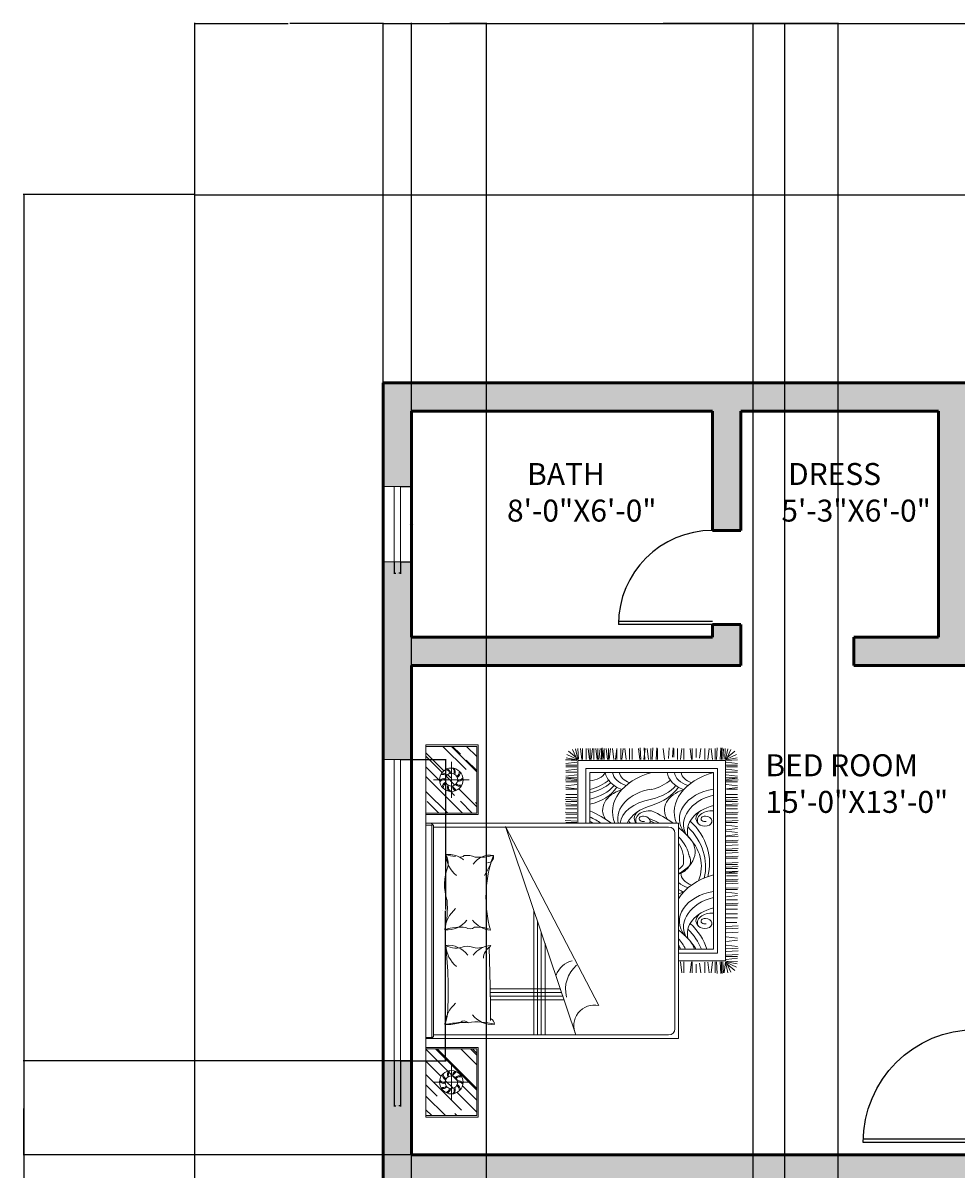
# Model space of a CAD drawing. Units: inches. Extents: x 134045 to 134755, y 144691 to 145880.
# Tile 4 of 6: x 134045 to 134343, y 145515 to 145880. Entities that reach past the tile are written whole.
import ezdxf

# ---------------------------------------------------------------- set-up
doc = ezdxf.new("R2010")
doc.units = ezdxf.units.IN
for name, color, linetype, lineweight in [('A-ANNO-DIMS', 2, 'Continuous', 18), ('A-AREA-IDEN', 7, 'Continuous', 18), ('A-DOOR', 4, 'Continuous', 25), ('A-FURN', 8, 'Continuous', 18), ('A-GLAZ', 4, 'Continuous', 18), ('A-WALL', 7, 'Continuous', 50), ('A-WALL-PATT', 252, 'Continuous', 13), ('C-PROP', 7, 'Continuous', 25)]:
    doc.layers.add(name, color=color, linetype=linetype, lineweight=lineweight)
doc.styles.get("Standard").update_dxf_attribs({"font": 'arial.ttf'})
doc.dimstyles.get("Standard").update_dxf_attribs({"dimtxt": 0.18, "dimasz": 0.18, "dimexe": 0.18, "dimexo": 0.0625, "dimgap": 0.09, "dimtad": 0, "dimtih": 1, "dimtoh": 1, "dimdec": 4, "dimzin": 0, "dimdsep": 46, "dimtxsty": 'Standard', "dimcen": 0.09, "dimadec": 0, "dimazin": 0, "dimtfac": 1, "dimtdec": 4, "dimtofl": 0, "dimtmove": 0, "dimatfit": 3, "dimfxl": 1, "dimtolj": 1, "dimtzin": 0, "dimarcsym": 0})

# ---------------------------------------------------------------- blocks, each defined once
blk = doc.blocks.new('A$C64B41DC1')
for p, q in [((0, 2.5079), (2.9903, 2.5079)), ((0, 2.0879), (0, 2.5079)), ((0.012, 2.4618), (0.0581, 2.5079)), ((0.012, 2.3515), (0.1684, 2.5079)), ((0.012, 2.0999), (0.012, 2.5079)), ((0.0543, 2.2213), (0.3409, 2.5079)), ((0.1689, 2.4179), (0.2589, 2.5079)), ((0.3265, 2.386), (0.4484, 2.5079)), ((0.3699, 2.3332), (0.5445, 2.5079)), ((0.548, 2.5079), (0.548, 2.0999)), ((0.56, 2.5079), (0.56, 2.0879)), ((0.6301, 2.5079), (0.6301, 0.4779)), ((0.6401, 2.461), (0.6401, 2.5079)), ((0.6401, 2.5079), (2.344, 2.5079)), ((2.344, 2.5079), (2.3601, 2.5079)), ((2.344, 2.5079), (2.344, 2.461)), ((2.3601, 2.5079), (2.3601, 2.4761)), ((2.3601, 0.4779), (2.3601, 2.5079)), ((2.4303, 2.5079), (2.4303, 2.0879)), ((2.4423, 2.5079), (2.4423, 2.0999)), ((2.4423, 2.3333), (2.6169, 2.5079)), ((2.4423, 2.2145), (2.7357, 2.5079)), ((2.4423, 2.404), (2.5354, 2.4971)), ((2.705, 2.398), (2.8149, 2.5079)), ((2.7691, 2.3772), (2.8998, 2.5079)), ((2.7819, 2.3646), (2.9252, 2.5079)), ((2.9783, 2.0999), (2.9783, 2.5079)), ((2.9903, 2.0879), (2.9903, 2.5079)), ((0.2157, 2.0999), (0.548, 2.4322)), ((0.2299, 2.0999), (0.548, 2.418)), ((0.2804, 2.1597), (0.2804, 2.4481)), ((2.344, 2.461), (0.6401, 2.461)), ((0.6601, 2.4461), (1.4951, 2.4461)), ((0.6601, 2.4461), (0.6601, 0.5579)), ((1.4951, 2.4461), (0.6697, 2.4461)), ((2.3301, 2.4461), (1.4951, 2.4461)), ((2.3301, 0.5579), (2.3301, 2.4461)), ((2.7099, 2.1597), (2.7099, 2.4481)), ((0.1362, 2.3039), (0.4246, 2.3039)), ((0.2311, 2.2906), (0.2937, 2.3532)), ((0.3405, 2.3039), (0.3605, 2.3238)), ((2.8541, 2.3039), (2.5657, 2.3039)), ((2.5849, 2.2779), (2.6158, 2.3088)), ((2.6158, 2.3088), (2.6313, 2.3243)), ((2.6674, 2.2756), (2.7382, 2.3464)), ((2.7249, 2.3076), (2.7512, 2.3339)), ((2.7746, 2.0999), (2.9783, 2.3036)), ((2.7914, 2.1846), (2.9783, 2.3715)), ((0.012, 2.261), (0.0275, 2.2765)), ((0.0404, 2.0999), (0.1982, 2.2578)), ((0.1365, 2.0999), (0.251, 2.2144)), ((0.2905, 2.2539), (0.3304, 2.2938)), ((0.4194, 2.0999), (0.548, 2.2285)), ((2.4423, 2.1353), (2.5382, 2.2312)), ((2.4918, 2.0999), (2.6366, 2.2447)), ((2.9144, 2.2312), (2.9783, 2.2951)), ((0.4986, 2.0999), (0.548, 2.1493)), ((0.5127, 2.0999), (0.548, 2.1352)), ((2.7831, 2.0999), (2.8678, 2.1846)), ((2.8962, 2.0999), (2.9783, 2.182)), ((0.56, 2.0879), (0, 2.0879)), ((0.548, 2.0999), (0.012, 2.0999)), ((2.4303, 2.0879), (2.9903, 2.0879)), ((2.4423, 2.0999), (2.9783, 2.0999)), ((2.5172, 2.0999), (2.5269, 2.1096)), ((0.9415, 1.9902), (0.9415, 1.3975)), ((0.9715, 1.9906), (0.9715, 1.4076)), ((1.0015, 1.991), (1.0015, 1.4177)), ((1.0315, 1.9916), (1.0315, 1.4279)), ((2.3349, 1.8678), (0.6613, 1.3029)), ((0.8956, 1.1191), (2.3349, 1.8678)), ((1.6636, 1.6412), (0.6601, 1.6412)), ((1.5748, 1.6112), (0.6601, 1.6112)), ((2.3665, 1.295), (2.3665, 1.3839)), ((2.377, 1.295), (2.3822, 1.3891)), ((2.4032, 1.295), (2.4032, 1.3839)), ((2.4346, 1.295), (2.4346, 1.3839)), ((2.4451, 1.295), (2.4503, 1.3891)), ((2.4774, 1.2957), (2.4774, 1.3837)), ((2.5, 1.295), (2.5, 1.3839)), ((2.5105, 1.295), (2.5157, 1.3891)), ((2.5367, 1.295), (2.5367, 1.3839)), ((2.5471, 1.295), (2.5524, 1.3891)), ((2.5681, 1.295), (2.5681, 1.3839)), ((2.5918, 1.295), (2.5918, 1.3839)), ((2.6346, 1.2957), (2.6346, 1.3837)), ((2.6362, 1.2957), (2.6467, 1.3839)), ((2.6729, 1.295), (2.6624, 1.3839)), ((2.6938, 1.295), (2.6938, 1.3839)), ((2.7043, 1.295), (2.7095, 1.3891)), ((2.7127, 1.2957), (2.7232, 1.3839)), ((2.7253, 1.295), (2.7253, 1.3839)), ((2.7494, 1.295), (2.7389, 1.3839)), ((2.7718, 1.295), (2.7718, 1.3839)), ((2.7959, 1.295), (2.7854, 1.3839)), ((2.8146, 1.2957), (2.8146, 1.3837)), ((2.8146, 1.2957), (2.8146, 1.3837)), ((2.8282, 1.295), (2.8282, 1.3839)), ((2.8282, 1.295), (2.8282, 1.3839)), ((2.8523, 1.295), (2.8418, 1.3839)), ((2.8523, 1.295), (2.8418, 1.3839)), ((2.8653, 1.2966), (2.8688, 1.3861)), ((2.8711, 1.2957), (2.8711, 1.3837)), ((2.8711, 1.2957), (2.8875, 1.3822)), ((2.8713, 1.2927), (2.954, 1.3315)), ((2.8717, 1.2884), (2.9588, 1.3058)), ((2.8765, 1.2958), (2.9132, 1.3758)), ((2.8893, 1.3011), (2.9394, 1.3636)), ((2.3601, 1.2873), (2.8639, 1.2873)), ((2.3601, 1.2233), (2.7999, 1.2233)), ((2.7999, 1.2233), (2.7999, 0.1658)), ((2.8639, 1.2873), (2.8639, 0.1018)), ((2.8716, 1.2565), (2.9605, 1.2669)), ((2.8716, 1.2212), (2.9605, 1.2212)), ((2.8716, 1.1947), (2.9605, 1.2052)), ((2.8723, 1.2489), (2.9603, 1.2489)), ((2.8744, 1.2817), (2.9603, 1.2869)), ((2.3601, 1.1913), (2.7679, 1.1912)), ((2.7679, 1.1912), (2.7679, 0.1978)), ((2.8716, 1.181), (2.9605, 1.1705)), ((2.8716, 1.1595), (2.9605, 1.1595)), ((2.8716, 1.133), (2.9605, 1.1435)), ((2.8716, 1.1193), (2.9605, 1.1088)), ((2.8723, 1.1872), (2.9603, 1.1872)), ((2.8723, 1.1255), (2.9603, 1.1255)), ((2.8716, 1.1035), (2.9605, 1.093)), ((2.8716, 1.0965), (2.9605, 1.0965)), ((2.8716, 1.086), (2.9657, 1.0913)), ((2.8716, 1.0756), (2.9605, 1.0756)), ((2.8716, 1.0491), (2.9605, 1.0596)), ((2.8716, 1.0354), (2.9605, 1.0249)), ((2.8723, 1.0858), (2.9605, 1.0753)), ((2.8723, 1.0416), (2.9603, 1.0416)), ((2.8716, 0.9346), (2.9605, 0.9241)), ((2.8723, 0.9987), (2.9605, 1.0092)), ((2.8723, 0.985), (2.9605, 0.9745)), ((2.8723, 0.9735), (2.9603, 0.9735)), ((2.8723, 0.9408), (2.9603, 0.9408)), ((2.8723, 0.8979), (2.9605, 0.9084)), ((2.8723, 0.8726), (2.9603, 0.8726)), ((2.8723, 0.8505), (2.9603, 0.8505)), ((2.8716, 0.7885), (2.9605, 0.799)), ((2.8716, 0.7818), (2.9657, 0.787)), ((2.8716, 0.7503), (2.9657, 0.7556)), ((2.8723, 0.7571), (2.9605, 0.7466)), ((2.8716, 0.7204), (2.9605, 0.7309)), ((2.8716, 0.6995), (2.9605, 0.6995)), ((2.8716, 0.689), (2.9657, 0.6838)), ((2.8716, 0.6576), (2.9657, 0.6523)), ((2.8716, 0.6471), (2.9605, 0.6471)), ((2.8716, 0.5903), (2.9605, 0.6007)), ((2.882, 0.5582), (2.9657, 0.5536)), ((0.6301, 0.4779), (2.3601, 0.4779)), ((0.7101, 0.5079), (2.2801, 0.5079)), ((1.2465, 0.4625), (1.1576, 0.452)), ((1.2542, 0.1018), (1.2542, 0.4779)), ((1.3182, 0.1658), (1.3182, 0.4779)), ((1.3502, 0.1978), (1.3502, 0.4779)), ((2.8716, 0.4877), (2.9603, 0.4877)), ((2.8716, 0.4625), (2.9605, 0.452)), ((2.8909, 0.5263), (2.9657, 0.5222)), ((2.8928, 0.5169), (2.9605, 0.5169)), ((1.2465, 0.3746), (1.1576, 0.3851)), ((1.2465, 0.4365), (1.1577, 0.4365)), ((1.2465, 0.3684), (1.1577, 0.3684)), ((2.8716, 0.4365), (2.9603, 0.4365)), ((2.8716, 0.3746), (2.9605, 0.3851)), ((2.8716, 0.3684), (2.9603, 0.3684)), ((1.2355, 0.3092), (1.1576, 0.3)), ((1.2285, 0.3357), (1.1577, 0.3357)), ((2.8826, 0.3092), (2.9605, 0.3)), ((2.8896, 0.3357), (2.9603, 0.3357)), ((1.2457, 0.2423), (1.1576, 0.2319)), ((1.2465, 0.2057), (1.1576, 0.2161)), ((1.2465, 0.1847), (1.1576, 0.1847)), ((1.2457, 0.2676), (1.1577, 0.2676)), ((2.7679, 0.1978), (1.3502, 0.1978)), ((2.8716, 0.2057), (2.9605, 0.2161)), ((2.8716, 0.1847), (2.9605, 0.1847)), ((2.8723, 0.2676), (2.9603, 0.2676)), ((2.8723, 0.2423), (2.9605, 0.2319)), ((1.2465, 0.1742), (1.1524, 0.169)), ((1.2465, 0.1428), (1.1524, 0.1376)), ((1.2465, 0.1334), (1.1524, 0.1281)), ((1.2465, 0.1323), (1.1576, 0.1323)), ((1.2465, 0.1323), (1.1576, 0.1323)), ((1.2465, 0.1), (1.1576, 0.1105)), ((1.2465, 0.1229), (1.1588, 0.1168)), ((1.2464, 0.1007), (1.1592, 0.0833)), ((1.2468, 0.0964), (1.1641, 0.0576)), ((1.2415, 0.0933), (1.2049, 0.0133)), ((1.247, 0.0934), (1.2306, 0.0069)), ((1.2527, 0.0925), (1.2493, 0.003)), ((2.8639, 0.1018), (1.2542, 0.1018)), ((1.2658, 0.0941), (1.2762, 0.0052)), ((1.2899, 0.0941), (1.2899, 0.0052)), ((1.2999, 0.0941), (1.3051, 0)), ((2.7999, 0.1658), (1.3182, 0.1658)), ((1.3313, 0.0941), (1.3365, 0)), ((1.3523, 0.0941), (1.3575, 0)), ((1.3804, 0.0941), (1.3699, 0.0052)), ((1.4119, 0.0934), (1.4223, 0.0052)), ((1.4485, 0.0941), (1.438, 0.0052)), ((1.48, 0.0941), (1.4852, 0)), ((1.5114, 0.0941), (1.5166, 0)), ((1.5323, 0.0941), (1.5376, 0)), ((1.5638, 0.0941), (1.5638, 0.0105)), ((1.6021, 0.0941), (1.6021, 0.0052)), ((1.6336, 0.0941), (1.6336, 0.0052)), ((1.6702, 0.0941), (1.6702, 0.0052)), ((1.7017, 0.0941), (1.7017, 0.0052)), ((1.7122, 0.0941), (1.7174, 0)), ((1.7445, 0.0934), (1.7445, 0.0054)), ((1.7698, 0.0934), (1.7803, 0.0052)), ((1.8065, 0.0941), (1.796, 0.0052)), ((1.8274, 0.0941), (1.8274, 0.0052)), ((1.8379, 0.0941), (1.8431, 0)), ((1.8746, 0.0941), (1.8798, 0)), ((1.8955, 0.0941), (1.8955, 0.0052)), ((1.906, 0.0941), (1.9113, 0)), ((1.9384, 0.0934), (1.9384, 0.0054)), ((1.9609, 0.0941), (1.9609, 0.0052)), ((1.9636, 0.0934), (1.9741, 0.0052)), ((1.9714, 0.0941), (1.9766, 0)), ((1.9976, 0.0941), (1.9976, 0.0052)), ((2.0081, 0.0941), (2.0133, 0)), ((2.029, 0.0941), (2.029, 0.0052)), ((2.0395, 0.0941), (2.0447, 0)), ((2.0797, 0.0941), (2.0797, 0.0052)), ((2.0902, 0.0941), (2.0954, 0)), ((2.1216, 0.0941), (2.1269, 0)), ((2.1412, 0.0941), (2.1412, 0.0052)), ((2.1517, 0.0941), (2.1569, 0)), ((2.1831, 0.0941), (2.1884, 0)), ((2.2093, 0.0941), (2.2093, 0.0052)), ((2.2198, 0.0941), (2.225, 0)), ((2.2512, 0.0941), (2.2565, 0)), ((2.2603, 0.0934), (2.2707, 0.0052)), ((2.2969, 0.0941), (2.2864, 0.0052)), ((2.3089, 0.0934), (2.3193, 0.0052)), ((2.3455, 0.0941), (2.3351, 0.0052)), ((2.3665, 0.0941), (2.3665, 0.0052)), ((2.377, 0.0941), (2.3822, 0)), ((2.4032, 0.0941), (2.4032, 0.0052)), ((2.4346, 0.0941), (2.4346, 0.0052)), ((2.4451, 0.0941), (2.4503, 0)), ((2.4774, 0.0934), (2.4774, 0.0054)), ((2.5, 0.0941), (2.5, 0.0052)), ((2.5105, 0.0941), (2.5157, 0)), ((2.5367, 0.0941), (2.5367, 0.0052)), ((2.5471, 0.0941), (2.5524, 0)), ((2.5681, 0.0941), (2.5681, 0.0052)), ((2.5918, 0.0941), (2.5918, 0.0052)), ((2.6346, 0.0934), (2.6346, 0.0054)), ((2.6362, 0.0934), (2.6467, 0.0052)), ((2.6729, 0.0941), (2.6624, 0.0052)), ((2.6938, 0.0941), (2.6938, 0.0052)), ((2.7043, 0.0941), (2.7095, 0)), ((2.7127, 0.0934), (2.7232, 0.0052)), ((2.7253, 0.0941), (2.7253, 0.0052)), ((2.7494, 0.0941), (2.7389, 0.0052)), ((2.7718, 0.0941), (2.7718, 0.0052)), ((2.7959, 0.0941), (2.7854, 0.0052)), ((2.8146, 0.0934), (2.8146, 0.0054)), ((2.8282, 0.0941), (2.8282, 0.0052)), ((2.8523, 0.0941), (2.8418, 0.0052)), ((2.8653, 0.0925), (2.8688, 0.003)), ((2.8711, 0.0934), (2.8875, 0.0069)), ((2.8713, 0.0964), (2.954, 0.0576)), ((2.8716, 0.1742), (2.9657, 0.169)), ((2.8716, 0.1428), (2.9657, 0.1376)), ((2.8716, 0.1334), (2.9657, 0.1281)), ((2.8716, 0.1323), (2.9605, 0.1323)), ((2.8716, 0.1229), (2.9593, 0.1168)), ((2.8717, 0.1007), (2.9588, 0.0833)), ((2.8744, 0.1074), (2.9603, 0.1022)), ((2.8765, 0.0933), (2.9132, 0.0133)), ((1.2288, 0.088), (1.1787, 0.0255)), ((2.8893, 0.088), (2.9394, 0.0255))]:
    blk.add_line(p, q)
at = {"ltscale": 10}
for p, q in [((1.4859, 1.5812), (0.6601, 1.5812)), ((1.397, 1.5512), (0.6601, 1.5512))]:
    blk.add_line(p, q, dxfattribs=at)
for centre, radius in [((0.2804, 2.3039), 0.0942), ((2.7099, 2.3039), 0.0942), ((0.2804, 2.3039), 0.051), ((2.7099, 2.3039), 0.051)]:
    blk.add_circle(centre, radius)
for centre, radius, start, end in [((0.3286, 2.3561), 0.0605, 136.17003, 182.48975), ((0.3231, 2.3585), 0.0462, 124.30017, 184.53802), ((0.6601, 2.4761), 0.03, 180, 270), ((2.3301, 2.4761), 0.03, 270, 0), ((2.6672, 2.3585), 0.0462, 355.46198, 55.69983), ((2.6617, 2.3561), 0.0605, 357.51025, 43.82997), ((0.2457, 2.3659), 0.0605, 208.17003, 254.48975), ((0.2417, 2.3614), 0.0462, 196.30017, 256.53802), ((0.2887, 2.3745), 0.0605, 172.17003, 218.48975), ((0.2828, 2.3731), 0.0462, 160.30017, 220.53802), ((0.3501, 2.3178), 0.0605, 100.17003, 146.48975), ((0.347, 2.323), 0.0462, 88.30017, 148.53802), ((0.3449, 2.2742), 0.0605, 64.17003, 110.48975), ((0.3455, 2.2802), 0.0462, 52.30017, 112.53802), ((1.0526, 2.3302), 0.3085, 175.30484, 198.69419), ((-0.8702, 2.0941), 1.6364, 4.80985, 9.18918), ((0.8579, 2.6278), 0.2948, 247.51785, 264.26696), ((0.728, 2.111), 0.245, 40.4189, 85.9871), ((1.0164, 5.7096), 3.3803, 266.81337, 276.16021), ((1.3963, 2.1044), 0.245, 94.0129, 139.5811), ((1.1858, 2.3288), 0.1943, 306.5711, 5.88998), ((1.5348, 2.2652), 0.1767, 151.77364, 201.69827), ((1.6986, 2.3355), 0.1943, 174.11002, 233.4289), ((1.1481, 2.2311), 0.3783, 353.49469, 19.18669), ((1.6871, 3.192), 0.8561, 257.74383, 273.62843), ((1.4882, 2.111), 0.245, 40.4189, 85.9871), ((1.8674, 1.9709), 0.3878, 68.20259, 108.9817), ((2.1269, 2.1044), 0.245, 94.0129, 139.5811), ((2.0342, 2.4856), 0.1563, 261.59582, 298.90918), ((1.9165, 2.3288), 0.1943, 333.73715, 5.88998), ((2.6058, 2.2028), 0.517, 163.60457, 172.3273), ((2.6448, 2.2802), 0.0462, 67.46198, 127.69983), ((2.6454, 2.2742), 0.0605, 69.51025, 115.82997), ((2.6433, 2.323), 0.0462, 31.46198, 91.69983), ((2.6402, 2.3178), 0.0605, 33.51025, 79.82997), ((2.7075, 2.3731), 0.0462, 319.46198, 19.69983), ((2.7016, 2.3745), 0.0605, 321.51025, 7.82997), ((2.7486, 2.3614), 0.0462, 283.46198, 343.69983), ((2.7446, 2.3659), 0.0605, 285.51025, 331.82997), ((0.2153, 2.3276), 0.0462, 232.30017, 292.53802), ((0.2158, 2.3336), 0.0605, 244.17003, 290.48975), ((0.2138, 2.2848), 0.0462, 268.30017, 328.53802), ((0.2107, 2.29), 0.0605, 280.17003, 326.48975), ((0.2377, 2.2493), 0.0462, 304.30017, 4.53802), ((0.2322, 2.2517), 0.0605, 316.17003, 2.48975), ((0.2779, 2.2347), 0.0462, 340.30017, 40.53802), ((0.272, 2.2333), 0.0605, 352.17003, 38.48975), ((0.3191, 2.2464), 0.0462, 16.30017, 76.53802), ((0.3151, 2.2419), 0.0605, 28.17003, 74.48975), ((0.7274, 2.2013), 0.0446, 314.4736, 42.17134), ((-1.6008, 2.277), 2.3618, 357.39054, 358.88764), ((1.9165, 2.3288), 0.1943, 320.94042, 333.73715), ((2.1347, 2.2313), 0.0459, 165.35061, 223.26844), ((2.6752, 2.2419), 0.0605, 105.51025, 151.82997), ((2.6712, 2.2464), 0.0462, 103.46198, 163.69983), ((2.7182, 2.2333), 0.0605, 141.51025, 187.82997), ((2.7123, 2.2347), 0.0462, 139.46198, 199.69983), ((2.7581, 2.2517), 0.0605, 177.51025, 223.82997), ((2.7526, 2.2493), 0.0462, 175.46198, 235.69983), ((2.7796, 2.29), 0.0605, 213.51025, 259.82997), ((2.7765, 2.2848), 0.0462, 211.46198, 271.69983), ((2.7744, 2.3336), 0.0605, 249.51025, 295.82997), ((2.775, 2.3276), 0.0462, 247.46198, 307.69983), ((0.9385, 1.978), 0.1943, 126.5711, 185.88998), ((0.2688, 2.0945), 0.4956, 344.0243, 8.70709), ((1.1858, 1.9714), 0.1943, 4.31813, 53.4289), ((1.204, 2.1778), 0.1681, 337.01697, 7.53676), ((1.7059, 1.9714), 0.204, 127.11975, 175.09005), ((1.5671, 2.1546), 0.0547, 142.08329, 220.902), ((1.1965, 2.0983), 0.3299, 343.79543, 3.55541), ((1.9394, 1.991), 0.1651, 351.26213, 55.75721), ((1.9346, 2.1778), 0.1681, 337.01697, 7.53676), ((1.2687, 1.9248), 0.1223, 33.62799, 86.47438), ((1.5415, 2.0969), 0.1834, 175.22328, 196.23004), ((1.7676, 1.0629), 0.9631, 69.65065, 105.96307), ((2.2748, 2.5795), 0.6373, 238.34989, 254.31375), ((2.4617, 2.0719), 0.3745, 173.82958, 196.4356), ((0.7417, 2.0149), 0.057, 273.47085, 328.54118), ((0.728, 2.2025), 0.245, 274.0129, 278.34166), ((0.7246, 18.8439), 16.8552, 270.17399, 272.05214), ((1.3401, 1.9404), 0.0603, 49.09906, 101.37023), ((2.0911, 2.0123), 0.0478, 179.77267, 283.80184), ((1.0274, 1.1334), 0.2527, 40.62904, 104.37123), ((1.0747, 1.2871), 0.1871, 14.1863, 69.12121), ((0.7347, 1.1553), 0.1649, 347.31088, 116.44537), ((0.7101, 0.5579), 0.05, 180, 270), ((2.2801, 0.5579), 0.05, 270, 0)]:
    blk.add_arc(centre, radius, start, end)
for centre, major_axis, ratio, start_param, end_param in [((1.9938, 1.6262), (0, -0.7531), 0.68, 0.797284, 0.954936), ((2.0643, 1.466), (0, -0.5322), 0.68, 7.239912, 7.311536), ((1.9052, 1.7397), (0, -0.9842), 0.68, 0.74745, 0.979724), ((2.4665, 0.8216), (0, -0.2664), 0.68, 2.006169, 3.565187), ((2.7455, 1.3081), (0, 0.3614), 0.68, 1.900046, 2.742661), ((2.7868, 1.3081), (0, 0.3614), 0.68, 1.900046, 2.614747), ((2.8372, 1.3081), (0, 0.3614), 0.68, 1.900046, 2.479658), ((2.8607, 1.3211), (0, 0.3614), 0.68, 1.938265, 2.479658), ((2.8057, 1.2079), (0, -0.1524), 0.68, 4.821745, 5.895886), ((2.4513, 0.5069), (0, 0.502), 0.68, 5.095327, 6.553458), ((2.7862, 0.8069), (0, -0.2615), 0.68, 3.244645, 4.205018), ((2.396, 0.6032), (0, 0.3641), 0.68, -1.3172, 0.145284), ((2.3507, 0.5642), (0.0073, 0.3819), 0.56205, -1.21172, -0.009991), ((2.7784, 0.8289), (0, -0.1802), 0.68, 3.227058, 4.318474), ((2.7821, 0.7971), (0, -0.1589), 0.68, 3.272942, 4.229533), ((2.2964, 0.5771), (0, -0.3263), 0.68, 1.938944, 2.850232), ((2.0403, 1.6015), (0, -0.8763), 0.68, 6.849801, 6.887077), ((2.4005, 0.7132), (0, -0.1214), 0.68, 2.284368, 3.652258), ((2.3834, 0.7081), (0, 0.1147), 0.68, 4.593909, 6.585576), ((2.3774, 0.7653), (0, -0.0593), 0.68, 5.841311, 7.755362), ((2.3961, 0.7628), (0, -0.0317), 0.68, 1.462497, 5.046281), ((1.9938, 1.1295), (-0.0678, 0.7439), 0.610498, 3.917146, 4.063997), ((2.0643, 0.9693), (0, -0.5322), 0.68, 7.239912, 7.336618), ((1.9052, 1.243), (0, -0.9842), 0.68, 0.74745, 0.979724), ((2.7455, 0.8114), (-0.0599, 0.3735), 0.695517, 1.775813, 2.548612), ((2.7868, 0.8114), (0, 0.3614), 0.68, 1.900046, 2.614747), ((2.8607, 0.8243), (0, 0.3614), 0.68, 1.938265, 2.479658), ((2.4513, 0.0102), (0, 0.502), 0.68, 5.095327, 6.553458), ((2.4665, 0.3249), (0, -0.2664), 0.68, 2.006169, 3.565187), ((2.7862, 0.3102), (0, -0.2615), 0.68, 3.244645, 4.205018), ((1.242, 0.9693), (0, -0.5322), 0.68, 6.586764, 6.677612), ((1.1714, 1.1295), (-0.1157, 0.7241), 0.59432, 3.291697, 3.50733), ((1.0828, 1.243), (0, -0.9842), 0.68, 0.565948, 0.680366), ((1.5283, 0.0674), (0, -0.3703), 0.68, 1.930561, 3.464283), ((1.5736, 0.1065), (0, 0.3641), 0.68, -1.3172, 0.476403), ((1.6289, 0.0102), (0, 0.502), 0.68, 6.655152, 6.661293), ((1.6289, 0.0102), (0, 0.502), 0.68, 5.095327, 5.911219), ((1.6442, 0.3249), (0, -0.2664), 0.68, 2.006169, 2.182797), ((1.9638, 0.3102), (0, -0.2615), 0.68, 4.015924, 4.205018), ((1.956, 0.3322), (0, -0.1802), 0.68, 3.770744, 4.318474), ((2.0606, 0.5616), (0, -0.1803), 0.68, 5.194792, 5.929328), ((2.0606, 0.5616), (0, -0.1803), 0.68, 5.194792, 6.723255), ((2.1315, 0.6603), (0, -0.3155), 0.68, 5.328638, 6.949396), ((2.0549, 0.5656), (0, -0.1303), 0.68, 5.450951, 6.054641), ((2.0643, 0.9693), (0, -0.5322), 0.68, 6.20013, 6.677612), ((1.9938, 1.1295), (-0.0678, 0.7439), 0.610498, 3.199135, 3.592282), ((1.9052, 1.243), (0, -0.9842), 0.68, 0.565948, 0.680366), ((2.3507, 0.0674), (0, -0.3703), 0.68, 1.930561, 3.464283), ((2.396, 0.1065), (0, 0.3641), 0.68, -1.3172, 0.476403), ((2.4513, 0.0102), (0, 0.502), 0.68, 6.655152, 6.661293), ((2.7784, 0.3322), (0, -0.1802), 0.68, 3.227058, 4.318474), ((1.1933, 0.9181), (0, -0.624), 0.68, 0.378672, 0.625379), ((1.3091, 0.6603), (0, -0.3155), 0.68, 6.475719, 6.949396), ((1.1911, 1.1066), (0, 0.8458), 0.68, 3.421828, 3.728616), ((1.2179, 1.1047), (0, -0.8763), 0.68, 6.507006, 6.887077), ((1.474, 0.0804), (0, -0.3263), 0.68, 1.938944, 3.339184), ((1.9597, 0.3004), (0, -0.1589), 0.68, 3.14258, 4.229533), ((2.0157, 0.9181), (0, -0.624), 0.68, -0.280078, 0.625379), ((2.0135, 1.1066), (0, 0.8458), 0.68, 2.978727, 3.728616), ((2.0403, 1.1047), (0, -0.8763), 0.68, 6.099302, 6.887077), ((2.2964, 0.0804), (0, -0.3263), 0.68, 1.938944, 3.339184), ((2.7821, 0.3004), (0, -0.1589), 0.68, 3.272942, 4.229533), ((1.555, 0.2685), (0, -0.0593), 0.68, 3.732151, 7.755362), ((1.5781, 0.2165), (0, -0.1214), 0.68, 2.284368, 3.726131), ((1.561, 0.2114), (0, 0.1147), 0.68, 4.593909, 6.647252), ((1.5737, 0.2661), (0, -0.0317), 0.68, 1.462497, 5.046281), ((2.3774, 0.2685), (0, -0.0593), 0.68, 3.732151, 7.755362), ((2.4005, 0.2165), (0, -0.1214), 0.68, 2.284368, 3.726131), ((2.3834, 0.2114), (0, 0.1147), 0.68, 4.593909, 6.647252), ((2.3961, 0.2661), (0, -0.0317), 0.68, 1.462497, 5.046281)]:
    blk.add_ellipse(centre, major_axis=major_axis, ratio=ratio, start_param=start_param, end_param=end_param)
blk = doc.blocks.new('DOOR-SWING-36IN')
for p, q in [((0, 1), (35.99, 1)), ((0, 0), (0, 1)), ((0, 0), (36, 0))]:
    blk.add_line(p, q)
blk.add_arc((0, 0), 36, 0, 90)
blk = doc.blocks.new('WIN-GLAZ-24IN')
for p, q in [((0, 0), (0, 24)), ((2, 0), (2, 24))]:
    blk.add_line(p, q)
blk = doc.blocks.new('WIN-GLAZ-96IN')
for p, q in [((0, 0), (0, 96)), ((2, 0), (2, 96))]:
    blk.add_line(p, q)
blk = doc.blocks.new('*D26')
at = {"layer": 'A-ANNO-DIMS', "color": 0, "lineweight": -2, "transparency": 16777216}
for p, q in [((134165.67, 145732.38), (134169.38, 145732.38)), ((134169.2, 145732.2), (134169.2, 145720.56)), ((134169.2, 145708.56), (134169.2, 145720.19)), ((134165.67, 145708.38), (134169.38, 145708.38))]:
    blk.add_line(p, q, dxfattribs=at)
at = {"layer": 'A-ANNO-DIMS', "color": 0, "transparency": 16777216}
for points in [[(134169.17, 145732.2), (134169.23, 145732.2), (134169.2, 145732.38)], [(134169.17, 145708.56), (134169.23, 145708.56), (134169.2, 145708.38)]]:
    blk.add_solid(points, dxfattribs=at)
at = {"layer": 'Defpoints', "color": 0, "transparency": 16777216}
for p in [(134165.6, 145732.38), (134169.2, 145732.38), (134165.6, 145708.38)]:
    blk.add_point(p, dxfattribs=at)
at = {"layer": 'A-ANNO-DIMS', "color": 0, "transparency": 16777216, "insert": (134169.2, 145720.38), "char_height": 0.18, "attachment_point": 5}
blk.add_mtext('\\A1;WINDOW 24 TYP.', dxfattribs=at)
blk = doc.blocks.new('*D27')
at = {"layer": 'A-ANNO-DIMS', "color": 0, "lineweight": -2, "transparency": 16777216}
for p, q in [((134163.6, 145708.31), (134163.6, 145704.6)), ((134165.6, 145708.31), (134165.6, 145704.6)), ((134163.78, 145704.78), (134164.14, 145704.78)), ((134165.42, 145704.78), (134165.06, 145704.78))]:
    blk.add_line(p, q, dxfattribs=at)
at = {"layer": 'A-ANNO-DIMS', "color": 0, "transparency": 16777216}
for points in [[(134163.78, 145704.81), (134163.78, 145704.75), (134163.6, 145704.78)], [(134165.42, 145704.81), (134165.42, 145704.75), (134165.6, 145704.78)]]:
    blk.add_solid(points, dxfattribs=at)
at = {"layer": 'Defpoints', "color": 0, "transparency": 16777216}
for p in [(134163.6, 145708.38), (134165.6, 145708.38), (134165.6, 145704.78)]:
    blk.add_point(p, dxfattribs=at)
at = {"layer": 'A-ANNO-DIMS', "color": 0, "transparency": 16777216, "insert": (134164.6, 145704.78), "char_height": 0.18, "attachment_point": 5}
blk.add_mtext('\\A1;2 TYP.', dxfattribs=at)
blk = doc.blocks.new('*D28')
at = {"layer": 'A-ANNO-DIMS', "color": 0, "lineweight": -2, "transparency": 16777216}
for p, q in [((134165.67, 145645.38), (134180.18, 145645.38)), ((134180, 145645.2), (134180, 145597.56)), ((134180, 145549.56), (134180, 145597.19)), ((134165.67, 145549.38), (134180.18, 145549.38))]:
    blk.add_line(p, q, dxfattribs=at)
at = {"layer": 'A-ANNO-DIMS', "color": 0, "transparency": 16777216}
for points in [[(134179.97, 145645.2), (134180.03, 145645.2), (134180, 145645.38)], [(134179.97, 145549.56), (134180.03, 145549.56), (134180, 145549.38)]]:
    blk.add_solid(points, dxfattribs=at)
at = {"layer": 'Defpoints', "color": 0, "transparency": 16777216}
for p in [(134165.6, 145645.38), (134180, 145645.38), (134165.6, 145549.38)]:
    blk.add_point(p, dxfattribs=at)
at = {"layer": 'A-ANNO-DIMS', "color": 0, "transparency": 16777216, "insert": (134180, 145597.38), "char_height": 0.18, "attachment_point": 5}
blk.add_mtext('\\A1;WINDOW 96 TYP.', dxfattribs=at)
blk = doc.blocks.new('*D29')
at = {"layer": 'A-ANNO-DIMS', "color": 0, "lineweight": -2, "transparency": 16777216}
for p, q in [((134163.6, 145549.31), (134163.6, 145534.8)), ((134165.6, 145549.31), (134165.6, 145534.8)), ((134163.78, 145534.98), (134164.14, 145534.98)), ((134165.42, 145534.98), (134165.06, 145534.98))]:
    blk.add_line(p, q, dxfattribs=at)
at = {"layer": 'A-ANNO-DIMS', "color": 0, "transparency": 16777216}
for points in [[(134163.78, 145535.01), (134163.78, 145534.95), (134163.6, 145534.98)], [(134165.42, 145535.01), (134165.42, 145534.95), (134165.6, 145534.98)]]:
    blk.add_solid(points, dxfattribs=at)
at = {"layer": 'Defpoints', "color": 0, "transparency": 16777216}
for p in [(134163.6, 145549.38), (134165.6, 145549.38), (134165.6, 145534.98)]:
    blk.add_point(p, dxfattribs=at)
at = {"layer": 'A-ANNO-DIMS', "color": 0, "transparency": 16777216, "insert": (134164.6, 145534.98), "char_height": 0.18, "attachment_point": 5}
blk.add_mtext('\\A1;2 TYP.', dxfattribs=at)
blk = doc.blocks.new('*D47')
at = {"layer": 'A-ANNO-DIMS', "color": 0, "lineweight": -2, "transparency": 16777216}
for p, q in [((134100.04, 145825.38), (134045.37, 145825.38)), ((134045.55, 145825.2), (134045.55, 145285.56)), ((134045.55, 144745.56), (134045.55, 145285.19)), ((134100.04, 144745.38), (134045.37, 144745.38))]:
    blk.add_line(p, q, dxfattribs=at)
at = {"layer": 'A-ANNO-DIMS', "color": 0, "transparency": 16777216}
for points in [[(134045.52, 145825.2), (134045.58, 145825.2), (134045.55, 145825.38)], [(134045.52, 144745.56), (134045.58, 144745.56), (134045.55, 144745.38)]]:
    blk.add_solid(points, dxfattribs=at)
at = {"layer": 'Defpoints', "color": 0, "transparency": 16777216}
for p in [(134045.55, 145825.38), (134100.1, 145825.38), (134100.1, 144745.38)]:
    blk.add_point(p, dxfattribs=at)
at = {"layer": 'A-ANNO-DIMS', "color": 0, "transparency": 16777216, "insert": (134045.55, 145285.38), "char_height": 0.18, "attachment_point": 5}
blk.add_mtext('\\A1;1080', dxfattribs=at)
blk = doc.blocks.new('*D48')
at = {"layer": 'A-ANNO-DIMS', "color": 0, "lineweight": -2, "transparency": 16777216}
for p, q in [((134160.1, 145765.44), (134160.1, 145880.11)), ((134160.28, 145879.93), (134399.81, 145879.93)), ((134639.92, 145879.93), (134400.4, 145879.93)), ((134640.1, 145765.44), (134640.1, 145880.11))]:
    blk.add_line(p, q, dxfattribs=at)
at = {"layer": 'A-ANNO-DIMS', "color": 0, "transparency": 16777216}
for points in [[(134160.28, 145879.96), (134160.28, 145879.9), (134160.1, 145879.93)], [(134639.92, 145879.96), (134639.92, 145879.9), (134640.1, 145879.93)]]:
    blk.add_solid(points, dxfattribs=at)
at = {"layer": 'Defpoints', "color": 0, "transparency": 16777216}
for p in [(134640.1, 145879.93), (134160.1, 145765.38), (134640.1, 145765.38)]:
    blk.add_point(p, dxfattribs=at)
at = {"layer": 'A-ANNO-DIMS', "color": 0, "transparency": 16777216, "insert": (134400.1, 145879.93), "char_height": 0.18, "attachment_point": 5}
blk.add_mtext('\\A1;480', dxfattribs=at)
blk = doc.blocks.new('*D50')
at = {"layer": 'A-ANNO-DIMS', "color": 0, "lineweight": -2, "transparency": 16777216}
for p, q in [((134100.1, 145825.44), (134100.1, 145880.11)), ((134100.28, 145879.93), (134129.88, 145879.93)), ((134159.92, 145879.93), (134130.32, 145879.93)), ((134160.1, 145765.44), (134160.1, 145880.11))]:
    blk.add_line(p, q, dxfattribs=at)
at = {"layer": 'A-ANNO-DIMS', "color": 0, "transparency": 16777216}
for points in [[(134100.28, 145879.96), (134100.28, 145879.9), (134100.1, 145879.93)], [(134159.92, 145879.96), (134159.92, 145879.9), (134160.1, 145879.93)]]:
    blk.add_solid(points, dxfattribs=at)
at = {"layer": 'Defpoints', "color": 0, "transparency": 16777216}
for p in [(134160.1, 145879.93), (134100.1, 145825.38), (134160.1, 145765.38)]:
    blk.add_point(p, dxfattribs=at)
at = {"layer": 'A-ANNO-DIMS', "color": 0, "transparency": 16777216, "insert": (134130.1, 145879.93), "char_height": 0.18, "attachment_point": 5}
blk.add_mtext('\\A1;60', dxfattribs=at)
blk = doc.blocks.new('*D55')
at = {"layer": 'A-ANNO-DIMS', "color": 0, "lineweight": -2, "transparency": 16777216}
for p, q in [((134278.1, 145094.44), (134278.1, 145880.11)), ((134278.28, 145879.93), (134282.89, 145879.93)), ((134287.92, 145879.93), (134283.31, 145879.93)), ((134288.1, 145094.44), (134288.1, 145880.11))]:
    blk.add_line(p, q, dxfattribs=at)
at = {"layer": 'A-ANNO-DIMS', "color": 0, "transparency": 16777216}
for points in [[(134278.28, 145879.96), (134278.28, 145879.9), (134278.1, 145879.93)], [(134287.92, 145879.96), (134287.92, 145879.9), (134288.1, 145879.93)]]:
    blk.add_solid(points, dxfattribs=at)
at = {"layer": 'Defpoints', "color": 0, "transparency": 16777216}
for p in [(134288.1, 145879.93), (134278.1, 145094.38), (134288.1, 145094.38)]:
    blk.add_point(p, dxfattribs=at)
at = {"layer": 'A-ANNO-DIMS', "color": 0, "transparency": 16777216, "insert": (134283.1, 145879.93), "char_height": 0.18, "attachment_point": 5}
blk.add_mtext('\\A1;10', dxfattribs=at)
blk = doc.blocks.new('*D71')
at = {"layer": 'A-ANNO-DIMS', "color": 0, "lineweight": -2, "transparency": 16777216}
for p, q in [((134169.1, 145283.44), (134169.1, 145880.11)), ((134169.28, 145879.93), (134180.88, 145879.93)), ((134192.92, 145879.93), (134181.32, 145879.93)), ((134193.1, 145307.44), (134193.1, 145880.11))]:
    blk.add_line(p, q, dxfattribs=at)
at = {"layer": 'A-ANNO-DIMS', "color": 0, "transparency": 16777216}
for points in [[(134169.28, 145879.96), (134169.28, 145879.9), (134169.1, 145879.93)], [(134192.92, 145879.96), (134192.92, 145879.9), (134193.1, 145879.93)]]:
    blk.add_solid(points, dxfattribs=at)
at = {"layer": 'Defpoints', "color": 0, "transparency": 16777216}
for p in [(134193.1, 145879.93), (134193.1, 145307.38), (134169.1, 145283.38)]:
    blk.add_point(p, dxfattribs=at)
at = {"layer": 'A-ANNO-DIMS', "color": 0, "transparency": 16777216, "insert": (134181.1, 145879.93), "char_height": 0.18, "attachment_point": 5}
blk.add_mtext('\\A1;24', dxfattribs=at)
blk = doc.blocks.new('*D72')
at = {"layer": 'A-ANNO-DIMS', "color": 0, "lineweight": -2, "transparency": 16777216}
for p, q in [((134193.1, 145307.44), (134193.1, 145880.11)), ((134193.28, 145879.93), (134248.82, 145879.93)), ((134304.92, 145879.93), (134249.38, 145879.93)), ((134305.1, 145307.44), (134305.1, 145880.11))]:
    blk.add_line(p, q, dxfattribs=at)
at = {"layer": 'A-ANNO-DIMS', "color": 0, "transparency": 16777216}
for points in [[(134193.28, 145879.96), (134193.28, 145879.9), (134193.1, 145879.93)], [(134304.92, 145879.96), (134304.92, 145879.9), (134305.1, 145879.93)]]:
    blk.add_solid(points, dxfattribs=at)
at = {"layer": 'Defpoints', "color": 0, "transparency": 16777216}
for p in [(134305.1, 145879.93), (134193.1, 145307.38), (134305.1, 145307.38)]:
    blk.add_point(p, dxfattribs=at)
at = {"layer": 'A-ANNO-DIMS', "color": 0, "transparency": 16777216, "insert": (134249.1, 145879.93), "char_height": 0.18, "attachment_point": 5}
blk.add_mtext('\\A1;112', dxfattribs=at)
blk = doc.blocks.new('*D73')
at = {"layer": 'A-ANNO-DIMS', "color": 0, "lineweight": -2, "transparency": 16777216}
for p, q in [((134169.04, 145549.38), (134045.37, 145549.38)), ((134045.55, 145549.2), (134045.55, 145534.56)), ((134045.55, 145519.56), (134045.55, 145534.19)), ((134169.04, 145519.38), (134045.37, 145519.38))]:
    blk.add_line(p, q, dxfattribs=at)
at = {"layer": 'A-ANNO-DIMS', "color": 0, "transparency": 16777216}
for points in [[(134045.52, 145549.2), (134045.58, 145549.2), (134045.55, 145549.38)], [(134045.52, 145519.56), (134045.58, 145519.56), (134045.55, 145519.38)]]:
    blk.add_solid(points, dxfattribs=at)
at = {"layer": 'Defpoints', "color": 0, "transparency": 16777216}
for p in [(134045.55, 145549.38), (134169.1, 145549.38), (134169.1, 145519.38)]:
    blk.add_point(p, dxfattribs=at)
at = {"layer": 'A-ANNO-DIMS', "color": 0, "transparency": 16777216, "insert": (134045.55, 145534.38), "char_height": 0.18, "attachment_point": 5}
blk.add_mtext('\\A1;30', dxfattribs=at)

msp = doc.modelspace()

# ---------------------------------------------------------------- hatches: boundary and pattern name
at = {"layer": 'A-WALL-PATT'}
h = msp.add_hatch(color=256, dxfattribs=at)
h.dxf.hatch_style = 1
h.paths.add_polyline_path([(134169.1037, 145756.3753), (134265.1037, 145756.3753), (134265.1037, 145718.3753), (134274.1037, 145718.3753), (134274.1037, 145756.3753), (134337.1037, 145756.3753), (134337.1037, 145684.3753), (134310.1037, 145684.3753), (134310.1037, 145675.3753), (134349.1037, 145675.3753), (134349.1037, 145559.3753), (134358.1037, 145559.3753), (134358.1037, 145598.3753), (134454.1037, 145598.3753), (134454.1037, 145590.3753), (134463.1037, 145590.3753), (134463.1037, 145635.3753), (134454.1037, 145635.3753), (134454.1037, 145603.3753), (134358.1037, 145603.3753), (134358.1037, 145675.3753), (134420.1037, 145675.3753), (134420.1037, 145684.3753), (134346.1037, 145684.3753), (134346.1037, 145756.3753), (134388.1037, 145756.3753), (134388.1037, 145765.3753), (134160.1037, 145765.3753), (134160.1037, 145732.3753), (134169.1037, 145732.3753)])
h = msp.add_hatch(color=256, dxfattribs=at)
h.dxf.hatch_style = 1
h.paths.add_polyline_path([(134274.1037, 145688.3753), (134265.1037, 145688.3753), (134265.1037, 145684.3753), (134169.1037, 145684.3753), (134169.1037, 145708.3753), (134160.1037, 145708.3753), (134160.1037, 145645.3753), (134169.1037, 145645.3753), (134169.1037, 145675.3753), (134274.1037, 145675.3753)])
h = msp.add_hatch(color=256, dxfattribs=at)
h.dxf.hatch_style = 1
h.paths.add_polyline_path([(134169.1037, 145427.3753), (134266.1037, 145427.3753), (134266.1037, 145432.3753), (134217.1037, 145432.3753), (134217.1037, 145436.3753), (134208.1037, 145436.3753), (134208.1037, 145432.3753), (134160.1037, 145432.3753), (134160.1037, 145374.4227), (134169.1037, 145374.4227)], flags=17)
h.paths.add_polyline_path([(134217.1037, 145479.3753), (134208.1037, 145479.3753), (134208.1037, 145472.3753), (134217.1037, 145472.3753)], flags=17)
h.paths.add_polyline_path([(134217.1037, 145510.3753), (134306.1037, 145510.3753), (134306.1037, 145432.3753), (134302.1037, 145432.3753), (134302.1037, 145427.3753), (134315.1037, 145427.3753), (134315.1037, 145432.3753), (134311.1037, 145432.3753), (134311.1037, 145510.3753), (134383.1037, 145510.3753), (134383.1037, 145432.3753), (134351.1037, 145432.3753), (134351.1037, 145427.3753), (134365.1037, 145427.3753), (134365.1037, 145343.3753), (134350.8634, 145329.135), (134357.2273, 145322.771), (134364.9677, 145330.5114), (134378.8831, 145316.5959), (134385.2471, 145322.9598), (134371.3316, 145336.8753), (134374.1037, 145339.6474), (134374.1037, 145427.3753), (134392.1037, 145427.3753), (134392.1037, 145519.3753), (134358.1037, 145519.3753), (134358.1037, 145523.3753), (134349.1037, 145523.3753), (134349.1037, 145519.3753), (134169.1037, 145519.3753), (134169.1037, 145549.3753), (134160.1037, 145549.3753), (134160.1037, 145510.3753), (134208.1037, 145510.3753), (134208.1037, 145503.3753), (134217.1037, 145503.3753)])

# ---------------------------------------------------------------- linework, layer by layer
at = {"layer": 'A-DOOR'}
for p, q in [((134265.1037, 145689.3753), (134235.1037, 145689.3753)), ((134265.1037, 145688.3753), (134235.1037, 145688.3753))]:
    msp.add_line(p, q, dxfattribs=at)
msp.add_arc((134265.1037, 145688.3753), 30, 90, 180, dxfattribs=at)
at = {"layer": 'A-GLAZ'}
for p, q in [((134169.1037, 145732.3753), (134160.1037, 145732.3753)), ((134169.1037, 145708.3753), (134160.1037, 145708.3753)), ((134169.1037, 145645.3753), (134160.1037, 145645.3753)), ((134169.1037, 145549.3753), (134160.1037, 145549.3753))]:
    msp.add_line(p, q, dxfattribs=at)
at = {"layer": 'A-WALL'}
for p, q in [((134160.1037, 145094.3753), (134160.1037, 145765.3753)), ((134160.1037, 145765.3753), (134640.1037, 145765.3753)), ((134169.1037, 145756.3753), (134265.1037, 145756.3753)), ((134169.1037, 145684.3753), (134169.1037, 145756.3753)), ((134265.1037, 145718.3753), (134265.1037, 145756.3753)), ((134274.1037, 145756.3753), (134337.1037, 145756.3753)), ((134274.1037, 145718.3753), (134274.1037, 145756.3753)), ((134337.1037, 145684.3753), (134337.1037, 145756.3753)), ((134265.1037, 145718.3753), (134274.1037, 145718.3753)), ((134265.1037, 145684.3753), (134265.1037, 145688.3753)), ((134265.1037, 145688.3753), (134274.1037, 145688.3753)), ((134274.1037, 145675.3753), (134274.1037, 145688.3753)), ((134169.1037, 145684.3753), (134265.1037, 145684.3753)), ((134310.1037, 145684.3753), (134337.1037, 145684.3753)), ((134310.1037, 145675.3753), (134310.1037, 145684.3753)), ((134169.1037, 145675.3753), (134274.1037, 145675.3753)), ((134169.1037, 145519.3753), (134169.1037, 145675.3753)), ((134310.1037, 145675.3753), (134349.1037, 145675.3753)), ((134169.1037, 145519.3753), (134349.1037, 145519.3753))]:
    msp.add_line(p, q, dxfattribs=at)
at = {"layer": 'C-PROP'}
for p, q in [((134100.1037, 145825.3753), (134700.1037, 145825.3753)), ((134100.1037, 144745.3753), (134100.1037, 145825.3753))]:
    msp.add_line(p, q, dxfattribs=at)

# ---------------------------------------------------------------- block references
at = {"layer": 'A-DOOR', "extrusion": (0, 0, -1), "zscale": -1}
msp.add_blockref('DOOR-SWING-36IN', (-134349.1034, 145523.375), dxfattribs=at)
at = {"layer": 'A-FURN', "xscale": 39.66398084585693, "yscale": 39.66398084585693, "zscale": 39.66398084585693, "rotation": 90}
msp.add_blockref('A$C64B41DC1', (134273.2291, 145531.4428), dxfattribs=at)
at = {"layer": 'A-GLAZ'}
for name, p in [('WIN-GLAZ-24IN', (134163.604, 145708.375)), ('WIN-GLAZ-96IN', (134163.604, 145549.375))]:
    msp.add_blockref(name, p, dxfattribs=at)

# ---------------------------------------------------------------- texts
at = {"layer": 'A-AREA-IDEN', "char_height": 7, "attachment_point": 1}
for s, width, insert in [('   BATH\\P8\'-0"X6\'-0"', 49.530184, (134199.5865, 145739.868)), (' DRESS\\P5\'-3"X6\'-0"', 49.530184, (134287.0359, 145739.868)), ('BED ROOM\\P15\'-0"X13\'-0"', 61.488508, (134281.9691, 145647.0489))]:
    msp.add_mtext_dynamic_manual_height_columns(s, width=width, gutter_width=12.5, heights=[0], dxfattribs=dict(at, insert=insert))

# ---------------------------------------------------------------- dimensions: what is measured, and where the dimension line sits
at = {"layer": 'A-ANNO-DIMS'}
for base, p1, p2, picture, middle in [((134160.1037, 145879.9253), (134100.1037, 145825.3753), (134160.1037, 145765.3753), '*D50', (134130.1037, 145879.9253)), ((134640.1037, 145879.9253), (134160.1037, 145765.3753), (134640.1037, 145765.3753), '*D48', (134400.1037, 145879.9253)), ((134193.1037, 145879.9253), (134169.1037, 145283.3753), (134193.1037, 145307.3753), '*D71', (134181.1037, 145879.9253)), ((134305.1037, 145879.9253), (134193.1037, 145307.3753), (134305.1037, 145307.3753), '*D72', (134249.1037, 145879.9253)), ((134288.1037, 145879.9253), (134278.1037, 145094.3753), (134288.1037, 145094.3753), '*D55', (134283.1037, 145879.9253))]:
    dim = msp.add_linear_dim(base=base, p1=p1, p2=p2, dimstyle='Standard', override={"dimdec": 0, "dimlfac": 1, "dimrnd": 0, "dimzin": 0, "dimdsep": 46, "dimlunit": 2}, dxfattribs=at)
    dim.commit()
    dim.dimension.update_dxf_attribs({"geometry": picture, "text_midpoint": middle})
for base, p1, p2, picture, middle in [((134045.5537, 145825.3753), (134100.1037, 144745.3753), (134100.1037, 145825.3753), '*D47', (134045.5537, 145285.3753)), ((134045.5537, 145549.3753), (134169.1037, 145519.3753), (134169.1037, 145549.3753), '*D73', (134045.5537, 145534.3753))]:
    dim = msp.add_linear_dim(base=base, p1=p1, p2=p2, angle=90, dimstyle='Standard', override={"dimdec": 0, "dimlfac": 1, "dimrnd": 0, "dimzin": 0, "dimdsep": 46, "dimlunit": 2}, dxfattribs=at)
    dim.commit()
    dim.dimension.update_dxf_attribs({"geometry": picture, "text_midpoint": middle})
for base, p1, p2, picture, middle in [((134169.2037, 145732.3753), (134165.6037, 145708.3753), (134165.6037, 145732.3753), '*D26', (134169.2037, 145720.3753)), ((134180.0037, 145645.3753), (134165.6037, 145549.3753), (134165.6037, 145645.3753), '*D28', (134180.0037, 145597.3753))]:
    dim = msp.add_linear_dim(base=base, p1=p1, p2=p2, angle=90, text='WINDOW <> TYP.', dimstyle='Standard', override={"dimdec": 0, "dimlfac": 1, "dimrnd": 0, "dimzin": 0, "dimdsep": 46, "dimlunit": 2}, dxfattribs=at)
    dim.commit()
    dim.dimension.update_dxf_attribs({"geometry": picture, "text_midpoint": middle})
for base, p1, p2, picture, middle in [((134165.6037, 145704.7753), (134163.6037, 145708.3753), (134165.6037, 145708.3753), '*D27', (134164.6037, 145704.7753)), ((134165.6037, 145534.9753), (134163.6037, 145549.3753), (134165.6037, 145549.3753), '*D29', (134164.6037, 145534.9753))]:
    dim = msp.add_linear_dim(base=base, p1=p1, p2=p2, text='<> TYP.', dimstyle='Standard', override={"dimdec": 0, "dimlfac": 1, "dimrnd": 0, "dimzin": 0, "dimdsep": 46, "dimlunit": 2}, dxfattribs=at)
    dim.commit()
    dim.dimension.update_dxf_attribs({"geometry": picture, "text_midpoint": middle})

doc.saveas('drawing.dxf')
